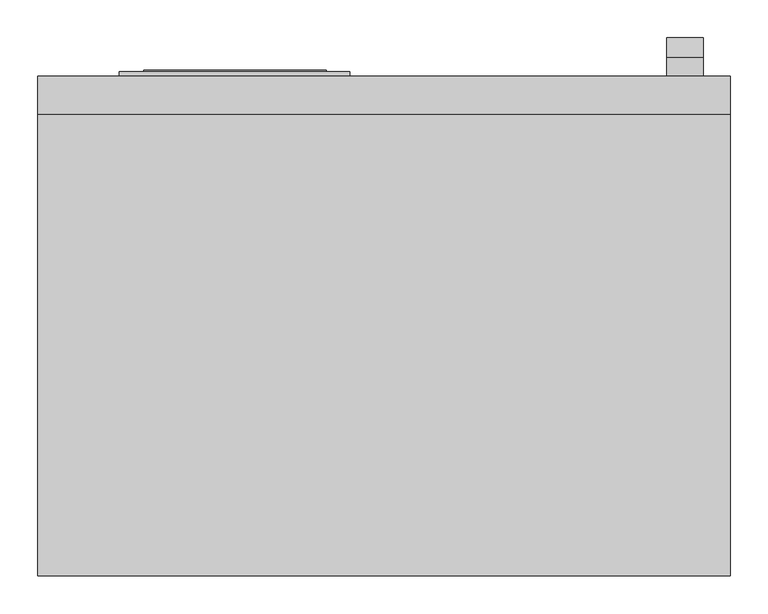
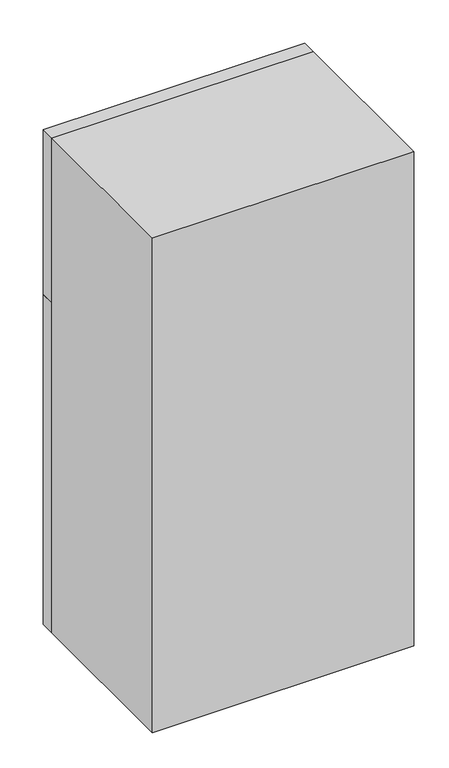
"""IFC4 building model written with IfcOpenShell, lengths in millimetres: furniture geometry."""

from ifc_helpers import new_model, si_unit, point, frame, frame_2d, origin, origin_with_axes, place, context, project, spatial, polyline, circle_curve, trimmed, segment, composite_curve, outline, extrude, faceted_brep, source, transform, mapped, element, save


def furniture_3f4f9d7a(model_context):
    return source(origin(), model_context, "Body", "SolidModel", [
        faceted_brep([(-154.8604727, 609.6, 0.0), (-1069.2604727, 609.6, 0.0), (-1069.2604727, 609.6, 1828.8), (-154.8604727, 609.6, 1828.8), (-983.107199, 609.6, 1745.9088241), (-983.107199, 609.6, 1288.7088241), (-221.107199, 609.6, 1288.7088241), (-221.107199, 609.6, 1745.9088241), (-983.107199, 609.6, 1168.6818903), (-983.107199, 609.6, 101.8818903), (-221.107199, 609.6, 101.8818903), (-221.107199, 609.6, 1168.6818903), (-154.8604727, 0.0, 0.0), (-154.8604727, 0.0, 1828.8), (-1069.2604727, 0.0, 1828.8), (-1069.2604727, 0.0, 0.0), (-221.107199, 101.6, 1745.9088241), (-221.107199, 101.6, 1288.7088241), (-983.107199, 101.6, 1288.7088241), (-983.107199, 101.6, 1745.9088241), (-221.107199, 101.6, 1168.6818903), (-221.107199, 101.6, 101.8818903), (-983.107199, 101.6, 101.8818903), (-983.107199, 101.6, 1168.6818903)], [[[0, 1, 2, 3], [4, 5, 6, 7], [8, 9, 10, 11]], [[12, 13, 14, 15]], [[3, 13, 12, 0]], [[2, 14, 13, 3]], [[1, 15, 14, 2]], [[0, 12, 15, 1]], [[16, 17, 18, 19]], [[19, 4, 7, 16]], [[18, 5, 4, 19]], [[17, 6, 5, 18]], [[16, 7, 6, 17]], [[20, 21, 22, 23]], [[23, 8, 11, 20]], [[22, 9, 8, 23]], [[21, 10, 9, 22]], [[20, 11, 10, 21]]]),
        extrude(outline(polyline([(-154.8604727, 660.4), (-154.8604727, 609.6), (-1069.2604727, 609.6), (-1069.2604727, 660.4), (-154.8604727, 660.4)])), frame((0.0, 0.0, 1220.3738546), z_axis=(0.0, 0.0, 1.0), x_axis=(1.0, 0.0, 0.0)), (0.0, 0.0, 1.0), 608.4261454),
        extrude(outline(polyline([(-154.8604727, 660.4), (-154.8604727, 609.6), (-1069.2604727, 609.6), (-1069.2604727, 660.4), (-154.8604727, 660.4)])), origin_with_axes(), (0.0, 0.0, 1.0), 1220.3738546),
        extrude(outline(composite_curve([segment(trimmed(circle_curve(frame_2d((685.8, 979.0738546)), 25.4), [point((685.8, 1004.4738546))], [point((711.2, 979.0738546))], False, "CARTESIAN"), True, "CONTINUOUS"), segment(polyline([(711.2, 979.0738546), (711.2, 426.6238546)]), True, "CONTINUOUS"), segment(trimmed(circle_curve(frame_2d((679.45, 426.6238546)), 31.75), [point((711.2, 426.6238546))], [point((679.45, 394.8738546))], False, "CARTESIAN"), True, "CONTINUOUS"), segment(polyline([(679.45, 394.8738546), (660.4, 394.8738546), (660.4, 420.2738546), (685.8, 420.2738546), (685.8, 979.0738546), (660.4, 979.0738546), (660.4, 1004.4738546), (685.8, 1004.4738546)]), True, "CONTINUOUS")], self_intersect=False)), frame((-238.6131994, 0.0, 0.0), z_axis=(1.0, 0.0, 0.0), x_axis=(0.0, 1.0, 0.0)), (0.0, 0.0, 1.0), 41.7631994),
        extrude(outline(composite_curve([segment(trimmed(circle_curve(frame_2d((685.8, 1714.1588241)), 25.4), [point((685.8, 1739.5588241))], [point((711.2, 1714.1588241))], False, "CARTESIAN"), True, "CONTINUOUS"), segment(polyline([(711.2, 1714.1588241), (711.2, 1333.1588241)]), True, "CONTINUOUS"), segment(trimmed(circle_curve(frame_2d((685.8, 1333.1588241)), 25.4), [point((711.2, 1333.1588241))], [point((685.8, 1307.7588241))], False, "CARTESIAN"), True, "CONTINUOUS"), segment(polyline([(685.8, 1307.7588241), (660.4, 1307.7588241), (660.4, 1333.1588241), (685.8, 1333.1588241), (685.8, 1714.1588241), (660.4, 1714.1588241), (660.4, 1739.5588241), (685.8, 1739.5588241)]), True, "CONTINUOUS")], self_intersect=False)), frame((-238.6131994, 0.0, 0.0), z_axis=(1.0, 0.0, 0.0), x_axis=(0.0, 1.0, 0.0)), (0.0, 0.0, 1.0), 48.1131994),
        extrude(outline(polyline([(-657.1290221, 666.75), (-657.1290221, 609.6), (-961.9290221, 609.6), (-961.9290221, 666.75), (-657.1290221, 666.75)])), frame((0.0, 0.0, 661.4796579), z_axis=(0.0, 0.0, 1.0), x_axis=(1.0, 0.0, 0.0)), (0.0, 0.0, 1.0), 304.8),
        extrude(outline(polyline([(-688.2162761, 668.3375), (-688.2162761, 648.467525), (-929.5162761, 648.467525), (-929.5162761, 668.3375), (-688.2162761, 668.3375)])), frame((0.0, 0.0, 700.7556373), z_axis=(0.0, 0.0, 1.0), x_axis=(1.0, 0.0, 0.0)), (0.0, 0.0, 1.0), 228.6),
    ])


if __name__ == "__main__":
    model = new_model("IFC4")
    model_context = context("Model", 3, world=origin())
    ifc_project = project(units=[si_unit("LENGTHUNIT", "METRE", prefix="MILLI")], contexts=[model_context])
    site = spatial("IfcSite", under=ifc_project)
    building = spatial("IfcBuilding", under=site)
    placement = place(None, origin())
    furniture_shape = furniture_3f4f9d7a(model_context)
    element("IfcFurniture", 1, at=placement, inside=building, context=model_context, shape_type="MappedRepresentation", body=[
        mapped(furniture_shape, transform((0.0, 0.0, 0.0), x_axis=(1.0, 0.0, 0.0), y_axis=(0.0, 1.0, 0.0), z_axis=(0.0, 0.0, 1.0))),
    ])
    save(model, "model.ifc")

# Revit data of these elements
# Type
#   Default Elevation = 0
# Element 1 (IfcFurniture)
#   Materials on its faces: "Default", "Default 3", "Default 2"
# Materials
#   "Default": colour RGB 127 127 127, transparency 0, Cost = 0
#   "Default 3": class "Glass", colour RGB 127 127 127, transparency 0
#   "Default 2": class "Plastic", colour RGB 127 127 127, transparency 0
